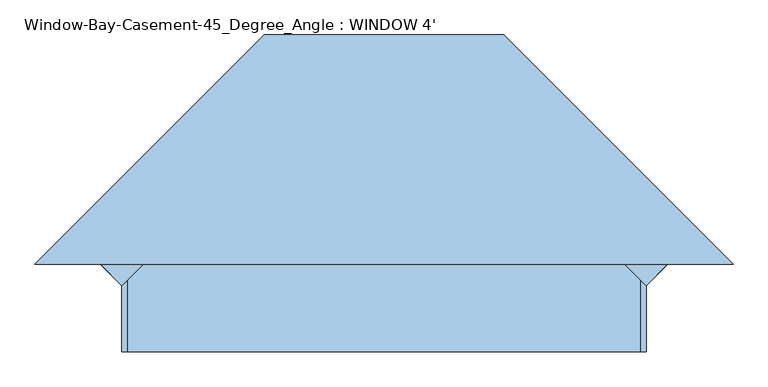
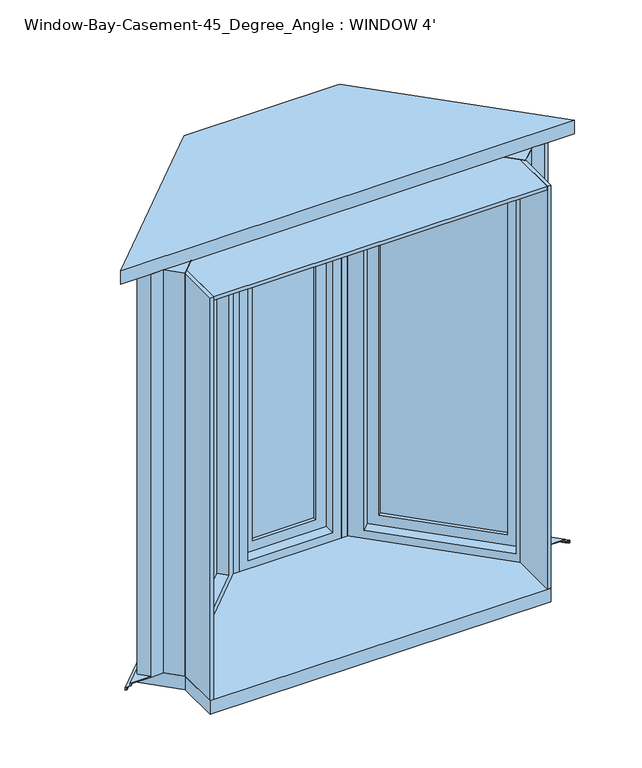
"""IFC4 building model written with IfcOpenShell, lengths in millimetres: window geometry, Window-Bay-Casement-45_Degree_Angle : WINDOW 4'."""

from ifc_helpers import new_model, si_unit, frame, origin, place, context, project, spatial, polyline, outline, extrude, faceted_brep, source, transform, mapped, element, save


def window_bay_casement_45_degree_angle_window_4_787d36ed(model_context):
    return source(origin(), model_context, "Body", "SolidModel", [
        extrude(outline(polyline([(609.6, 150.9914087), (605.1098719, 146.5012806), (314.3637138, 437.2474388), (318.8538418, 441.7375668), (609.6, 150.9914087)])), frame((0.0, 0.0, 730.25), z_axis=(0.0, 0.0, 1.0), x_axis=(1.0, 0.0, 0.0)), (0.0, 0.0, 1.0), 1384.3),
        extrude(outline(polyline([(600.6197439, 142.0111525), (596.1296158, 137.5210245), (305.3834576, 428.2671827), (309.8735857, 432.7573107), (600.6197439, 142.0111525)])), frame((0.0, 0.0, 730.25), z_axis=(0.0, 0.0, 1.0), x_axis=(1.0, 0.0, 0.0)), (0.0, 0.0, 1.0), 1384.3),
        extrude(outline(polyline([(1441.45, 57.15), (1441.45, -468.3271601), (-57.15, -468.3271601), (-57.15, 57.15), (1441.45, 57.15)]), holes=[polyline([(1384.3, -411.1771601), (1384.3, 0.0), (0.0, 0.0), (0.0, -411.1771601), (1384.3, -411.1771601)])]), frame((587.1493597, 128.5407684, 730.25), z_axis=(0.7071067811865468, 0.7071067811865483, 0.0), x_axis=(0.0, 0.0, 1.0)), (0.0, 0.0, 1.0), 44.45),
        faceted_brep([(204.6085913, 457.2, 2184.4), (609.6, 52.2085913, 2184.4), (658.9914087, 101.6, 2184.4), (703.8926893, 101.6, 2184.4), (246.6926893, 558.8, 2184.4), (627.5605122, 88.1296158, 2171.7), (255.992049, 459.6980791, 2171.7), (300.8933296, 504.5993597, 2171.7), (672.4617928, 133.0308964, 2171.7), (587.1493597, 74.6592316, 2152.65), (242.5216648, 419.2869265, 2152.65), (269.4624332, 446.2276949, 2152.65), (614.0901281, 101.6, 2152.65), (255.992049, 459.6980791, 673.1), (300.8933296, 504.5993597, 673.1), (242.5216648, 419.2869265, 692.15), (269.4624332, 446.2276949, 692.15), (246.6926893, 558.8, 660.4), (703.8926893, 101.6, 660.4), (658.9914087, 101.6, 660.4), (609.6, 52.2085913, 660.4), (204.6085913, 457.2, 660.4), (627.5605122, 88.1296158, 673.1), (672.4617928, 133.0308964, 673.1), (587.1493597, 74.6592316, 692.15), (614.0901281, 101.6, 692.15)], [[[0, 1, 2, 3, 4]], [[5, 6, 7, 8]], [[9, 10, 11, 12]], [[6, 13, 14, 7]], [[10, 15, 16, 11]], [[17, 18, 19, 20, 21]], [[13, 22, 23, 14]], [[15, 24, 25, 16]], [[20, 19, 2, 1]], [[3, 18, 17, 4], [7, 14, 23, 8]], [[8, 23, 22, 5]], [[5, 22, 13, 6], [11, 16, 25, 12]], [[12, 25, 24, 9]], [[1, 0, 21, 20], [9, 24, 15, 10]], [[4, 17, 21, 0]], [[2, 19, 18, 3]]]),
        extrude(outline(polyline([(-609.6, 150.9914087), (-318.8538418, 441.7375668), (-314.3637138, 437.2474388), (-605.1098719, 146.5012806), (-609.6, 150.9914087)])), frame((0.0, 0.0, 730.25), z_axis=(0.0, 0.0, 1.0), x_axis=(1.0, 0.0, 0.0)), (0.0, 0.0, 1.0), 1384.3),
        extrude(outline(polyline([(-600.6197439, 142.0111525), (-309.8735857, 432.7573107), (-305.3834576, 428.2671827), (-596.1296158, 137.5210245), (-600.6197439, 142.0111525)])), frame((0.0, 0.0, 730.25), z_axis=(0.0, 0.0, 1.0), x_axis=(1.0, 0.0, 0.0)), (0.0, 0.0, 1.0), 1384.3),
        extrude(outline(polyline([(1441.45, -57.15), (-57.15, -57.15), (-57.15, 468.3271601), (1441.45, 468.3271601), (1441.45, -57.15)]), holes=[polyline([(1384.3, 411.1771601), (0.0, 411.1771601), (0.0, 0.0), (1384.3, 0.0), (1384.3, 411.1771601)])]), frame((-587.1493597, 128.5407684, 730.25), z_axis=(-0.7071067811865468, 0.7071067811865483, 0.0), x_axis=(0.0, 0.0, 1.0)), (0.0, 0.0, 1.0), 44.45),
        faceted_brep([(-204.6085913, 457.2, 2184.4), (-246.6926893, 558.8, 2184.4), (-703.8926893, 101.6, 2184.4), (-658.9914087, 101.6, 2184.4), (-609.6, 52.2085913, 2184.4), (-627.5605122, 88.1296158, 2171.7), (-672.4617928, 133.0308964, 2171.7), (-300.8933296, 504.5993597, 2171.7), (-255.992049, 459.6980791, 2171.7), (-587.1493597, 74.6592316, 2152.65), (-614.0901281, 101.6, 2152.65), (-269.4624332, 446.2276949, 2152.65), (-242.5216648, 419.2869265, 2152.65), (-300.8933296, 504.5993597, 673.1), (-255.992049, 459.6980791, 673.1), (-269.4624332, 446.2276949, 692.15), (-242.5216648, 419.2869265, 692.15), (-246.6926893, 558.8, 660.4), (-204.6085913, 457.2, 660.4), (-609.6, 52.2085913, 660.4), (-658.9914087, 101.6, 660.4), (-703.8926893, 101.6, 660.4), (-672.4617928, 133.0308964, 673.1), (-627.5605122, 88.1296158, 673.1), (-614.0901281, 101.6, 692.15), (-587.1493597, 74.6592316, 692.15)], [[[0, 1, 2, 3, 4]], [[5, 6, 7, 8]], [[9, 10, 11, 12]], [[8, 7, 13, 14]], [[12, 11, 15, 16]], [[17, 18, 19, 20, 21]], [[14, 13, 22, 23]], [[16, 15, 24, 25]], [[19, 4, 3, 20]], [[2, 1, 17, 21], [7, 6, 22, 13]], [[6, 5, 23, 22]], [[5, 8, 14, 23], [11, 10, 24, 15]], [[10, 9, 25, 24]], [[4, 19, 18, 0], [9, 12, 16, 25]], [[1, 0, 18, 17]], [[3, 2, 21, 20]]]),
        faceted_brep([(-267.7347382, 609.6, 660.4), (-267.7347382, 609.6, 653.0697935), (267.7347382, 609.6, 653.0697935), (267.7347382, 609.6, 660.4), (-246.6926893, 558.8, 663.1486341), (-246.6926893, 558.8, 660.4), (246.6926893, 558.8, 660.4), (246.6926893, 558.8, 663.1486341), (-268.3133946, 610.997, 654.4483503), (-268.3133946, 610.997, 663.1486341), (268.3133946, 610.997, 663.1486341), (268.3133946, 610.997, 654.4483503), (273.5739068, 623.697, 652.2089977), (-273.5739068, 623.697, 652.2089977), (273.5739068, 623.697, 643.2668038), (-273.5739068, 623.697, 643.2668038), (-271.932627, 619.7346, 644.7270038), (-271.932627, 619.7346, 643.2668038), (271.932627, 619.7346, 643.2668038), (271.932627, 619.7346, 644.7270038), (-272.9110823, 622.0968, 650.8662705), (-272.9110823, 622.0968, 644.7270038), (272.9110823, 622.0968, 644.7270038), (272.9110823, 622.0968, 650.8662705), (-775.7347382, 101.6, 660.4), (-775.7347382, 101.6, 653.0697935), (775.7347382, 101.6, 660.4), (703.8926893, 101.6, 660.4), (-703.8926893, 101.6, 660.4), (-703.8926893, 101.6, 663.1486341), (703.8926893, 101.6, 663.1486341), (777.7103945, 101.6, 663.1486341), (-777.7103945, 101.6, 663.1486341), (-777.7103945, 101.6, 654.4483503), (-795.6709068, 101.6, 652.2089977), (-795.6709068, 101.6, 643.2668038), (795.6709068, 101.6, 643.2668038), (790.0672271, 101.6, 643.2668038), (-790.0672271, 101.6, 643.2668038), (-790.0672271, 101.6, 644.7270038), (790.0672271, 101.6, 644.7270038), (793.4078823, 101.6, 644.7270038), (-793.4078823, 101.6, 644.7270038), (-793.4078823, 101.6, 650.8662705), (775.7347382, 101.6, 653.0697935), (777.7103945, 101.6, 654.4483503), (795.6709068, 101.6, 652.2089977), (793.4078823, 101.6, 650.8662705)], [[[0, 1, 2, 3]], [[4, 5, 6, 7]], [[8, 9, 10, 11]], [[8, 11, 12, 13]], [[13, 12, 14, 15]], [[16, 17, 18, 19]], [[20, 21, 22, 23]], [[2, 1, 20, 23]], [[1, 0, 24, 25]], [[0, 3, 26, 27, 6, 5, 28, 24]], [[5, 4, 29, 28]], [[4, 7, 30, 31, 10, 9, 32, 29]], [[9, 8, 33, 32]], [[8, 13, 34, 33]], [[13, 15, 35, 34]], [[15, 14, 36, 37, 18, 17, 38, 35]], [[17, 16, 39, 38]], [[16, 19, 40, 41, 22, 21, 42, 39]], [[21, 20, 43, 42]], [[20, 1, 25, 43]], [[3, 2, 44, 26]], [[7, 6, 27, 30]], [[11, 10, 31, 45]], [[12, 11, 45, 46]], [[14, 12, 46, 36]], [[19, 18, 37, 40]], [[23, 22, 41, 47]], [[2, 23, 47, 44]], [[25, 24, 28, 29, 32, 33, 34, 35, 38, 39, 42, 43]], [[27, 26, 44, 47, 41, 40, 37, 36, 46, 45, 31, 30]]]),
        extrude(outline(polyline([(-681.442049, 124.0506403), (-703.8926893, 101.6), (-735.3235857, 133.0308964), (-712.8729454, 155.4815367), (-681.442049, 124.0506403)])), frame((0.0, 0.0, 663.1486341), z_axis=(0.0, 0.0, 1.0), x_axis=(1.0, 0.0, 0.0)), (0.0, 0.0, 1.0), 1521.2513659),
        extrude(outline(polyline([(681.442049, 124.0506403), (712.8729454, 155.4815367), (735.3235857, 133.0308964), (703.8926893, 101.6), (681.442049, 124.0506403)])), frame((0.0, 0.0, 663.1486341), z_axis=(0.0, 0.0, 1.0), x_axis=(1.0, 0.0, 0.0)), (0.0, 0.0, 1.0), 1521.2513659),
        extrude(outline(polyline([(278.2557627, 635.0), (811.6557627, 101.6), (-811.6557627, 101.6), (-278.2557627, 635.0), (278.2557627, 635.0)])), frame((0.0, 0.0, 2184.4), z_axis=(0.0, 0.0, 1.0), x_axis=(1.0, 0.0, 0.0)), (0.0, 0.0, 1.0), 50.8),
        extrude(outline(polyline([(-182.7414087, 558.8), (-182.7414087, 457.2), (-204.6085913, 457.2), (-246.6926893, 558.8), (-182.7414087, 558.8)])), frame((0.0, 0.0, 660.4), z_axis=(0.0, 0.0, 1.0), x_axis=(1.0, 0.0, 0.0)), (0.0, 0.0, 1.0), 1524.0),
        extrude(outline(polyline([(246.6926893, 558.8), (204.6085913, 457.2), (182.7414087, 457.2), (182.7414087, 558.8), (246.6926893, 558.8)])), frame((0.0, 0.0, 660.4), z_axis=(0.0, 0.0, 1.0), x_axis=(1.0, 0.0, 0.0)), (0.0, 0.0, 1.0), 1524.0),
        faceted_brep([(170.0414087, 495.3, 673.1), (170.0414087, 558.8, 673.1), (-170.0414087, 558.8, 673.1), (-170.0414087, 495.3, 673.1), (150.9914087, 457.2, 692.15), (150.9914087, 495.3, 692.15), (-150.9914087, 495.3, 692.15), (-150.9914087, 457.2, 692.15), (182.7414087, 558.8, 660.4), (182.7414087, 457.2, 660.4), (-182.7414087, 457.2, 660.4), (-182.7414087, 558.8, 660.4), (-170.0414087, 558.8, 2171.7), (-170.0414087, 495.3, 2171.7), (-150.9914087, 495.3, 2152.65), (-150.9914087, 457.2, 2152.65), (-182.7414087, 457.2, 2184.4), (-182.7414087, 558.8, 2184.4), (170.0414087, 558.8, 2171.7), (170.0414087, 495.3, 2171.7), (150.9914087, 495.3, 2152.65), (150.9914087, 457.2, 2152.65), (182.7414087, 457.2, 2184.4), (182.7414087, 558.8, 2184.4)], [[[0, 1, 2, 3]], [[4, 5, 6, 7]], [[8, 9, 10, 11]], [[3, 2, 12, 13]], [[7, 6, 14, 15]], [[11, 10, 16, 17]], [[13, 12, 18, 19]], [[15, 14, 20, 21]], [[17, 16, 22, 23]], [[11, 17, 23, 8], [1, 18, 12, 2]], [[19, 18, 1, 0]], [[3, 13, 19, 0], [5, 20, 14, 6]], [[21, 20, 5, 4]], [[9, 22, 16, 10], [7, 15, 21, 4]], [[23, 22, 9, 8]]]),
        extrude(outline(polyline([(112.8914087, 527.05), (112.8914087, 520.7), (-112.8914087, 520.7), (-112.8914087, 527.05), (112.8914087, 527.05)])), frame((0.0, 0.0, 730.25), z_axis=(0.0, 0.0, 1.0), x_axis=(1.0, 0.0, 0.0)), (0.0, 0.0, 1.0), 1384.3),
        extrude(outline(polyline([(112.8914087, 514.35), (112.8914087, 508.0), (-112.8914087, 508.0), (-112.8914087, 514.35), (112.8914087, 514.35)])), frame((0.0, 0.0, 730.25), z_axis=(0.0, 0.0, 1.0), x_axis=(1.0, 0.0, 0.0)), (0.0, 0.0, 1.0), 1384.3),
        extrude(outline(polyline([(609.6, -101.6), (-609.6, -101.6), (-609.6, 52.2085913), (-717.3630735, 159.9716648), (-267.7347382, 609.6), (267.7347382, 609.6), (717.3630735, 159.9716648), (609.6, 52.2085913), (609.6, -101.6)])), frame((0.0, 0.0, 609.6), z_axis=(0.0, 0.0, 1.0), x_axis=(1.0, 0.0, 0.0)), (0.0, 0.0, 1.0), 50.8),
        extrude(outline(polyline([(2171.7, -170.0414087), (673.1, -170.0414087), (673.1, 170.0414087), (2171.7, 170.0414087), (2171.7, -170.0414087)]), holes=[polyline([(2114.55, 112.8914087), (730.25, 112.8914087), (730.25, -112.8914087), (2114.55, -112.8914087), (2114.55, 112.8914087)])]), frame((0.0, 495.3, 0.0), z_axis=(0.0, 1.0, 0.0), x_axis=(0.0, 0.0, 1.0)), (0.0, 0.0, 1.0), 44.45),
        extrude(outline(polyline([(-609.6, -101.6), (-609.6, 52.2085913), (-596.9, 64.9085913), (-596.9, -101.6), (-609.6, -101.6)])), frame((0.0, 0.0, 660.4), z_axis=(0.0, 0.0, 1.0), x_axis=(1.0, 0.0, 0.0)), (0.0, 0.0, 1.0), 1524.0),
        extrude(outline(polyline([(609.6, -101.6), (596.9, -101.6), (596.9, 64.9085913), (609.6, 52.2085913), (609.6, -101.6)])), frame((0.0, 0.0, 660.4), z_axis=(0.0, 0.0, 1.0), x_axis=(1.0, 0.0, 0.0)), (0.0, 0.0, 1.0), 1524.0),
        extrude(outline(polyline([(-204.6085913, 457.2), (204.6085913, 457.2), (596.9, 64.9085913), (596.9, -101.6), (-596.9, -101.6), (-596.9, 64.9085913), (-204.6085913, 457.2)])), frame((0.0, 0.0, 2171.7), z_axis=(0.0, 0.0, 1.0), x_axis=(1.0, 0.0, 0.0)), (0.0, 0.0, 1.0), 12.7),
    ])


if __name__ == "__main__":
    model = new_model("IFC4")
    model_context = context("Model", 3, world=origin())
    ifc_project = project(units=[si_unit("LENGTHUNIT", "METRE", prefix="MILLI")], contexts=[model_context])
    site = spatial("IfcSite", under=ifc_project)
    building = spatial("IfcBuilding", under=site)
    placement = place(None, origin())
    window_bay_casement_45_degree_angle_window_4_shape = window_bay_casement_45_degree_angle_window_4_787d36ed(model_context)
    element("IfcWindow", 1, ObjectType="Window-Bay-Casement-45_Degree_Angle : WINDOW 4'", at=placement, inside=building, context=model_context, shape_type="MappedRepresentation", body=[
        mapped(window_bay_casement_45_degree_angle_window_4_shape, transform((0.0, 0.0, 0.0), x_axis=(1.0, 0.0, 0.0), y_axis=(0.0, 1.0, 0.0), z_axis=(0.0, 0.0, 1.0))),
    ])
    save(model, "model.ifc")

# Revit data of these elements
# Type "Window-Bay-Casement-45_Degree_Angle : WINDOW 4'"
#   Type Mark = "19"
#   Fire Rating = "0.5h"
#   Assembly Code = "B2020100"
#   Analytic Construction = "Double glazing - domestic"
#   Width of Middle Sash = 1' - 2.38909"
#   Width = 4' - 0"
#   Visual Light Transmittance = 0.81
#   Thermal Resistance (R) = 1.8146 (h·ft²·°F)/BTU
#   Solar Heat Gain Coefficient = 0.76
#   Rough Width = 4' - 0 1/2"
#   Rough Height = 5' - 0 1/2"
#   Length 4 = 0' - 1.13909"
#   Length 3 = 0' - 0.51777"
#   Length 2 = 1' - 7.42462"
#   Length 1 = 1' - 2.80546"
#   Wall Thickness [instance default] = 0' - 6"
#   Trim Width = 4' - 5.03553"
#   Trim Height = 5' - 0"
#   Height 1 = 5' - 2"
#   Height = 5' - 0"
#   Heat Transfer Coefficient (U) = 0.5511 BTU/(h·ft²·°F)
#   Depth = 1' - 6"
#   Default Sill Height = 2' - 0"
#   Angle 1 = 22.50°
#   Angle = 45.00°
#   Center Muntin Visibility = yes
#   Side Muntin Visibility = yes
#   Interior Trim Visibility [instance default] = yes
#   Exterior Trim Visibility [instance default] = yes
#   Center Muntin Pattern = Muntin Pattern_2x2 : Muntin Pattern_2x2
#   Side Muntin Pattern = Muntin Pattern_2x2 : Muntin Pattern_2x2
#   Interior Trim Material = Wood - Stained
#   Exterior Trim Material = Clad - White
#   Exterior Trim = element 406231
#   Interior Trim = Trim-Window-Interior-Flat : Picture Frame
#   Interior Frame Material = Wood - Stained
#   Glass Panel Material = Glass
#   Exterior Frame Material = Clad - White
#   Wall Closure = (empty or 0)
# Element 1 (IfcWindow, "Window-Bay-Casement-45_Degree_Angle : WINDOW 4'")
#   Wall Thickness = 0' - 8"
#   Materials on its faces: "Wood - Stained", "Clad - White", "Glass"
# Materials
#   "Wood - Stained": class "Wood", colour RGB 224 178 126, transparency 0, Cost = 0
#   "Clad - White": class "Wood", colour RGB 242 242 238, transparency 0, Cost = 0
#   "Glass": class "Glass", colour RGB 0 128 192, transparency 0.75, Description = "Soda Lime Glass", Cost = 0
